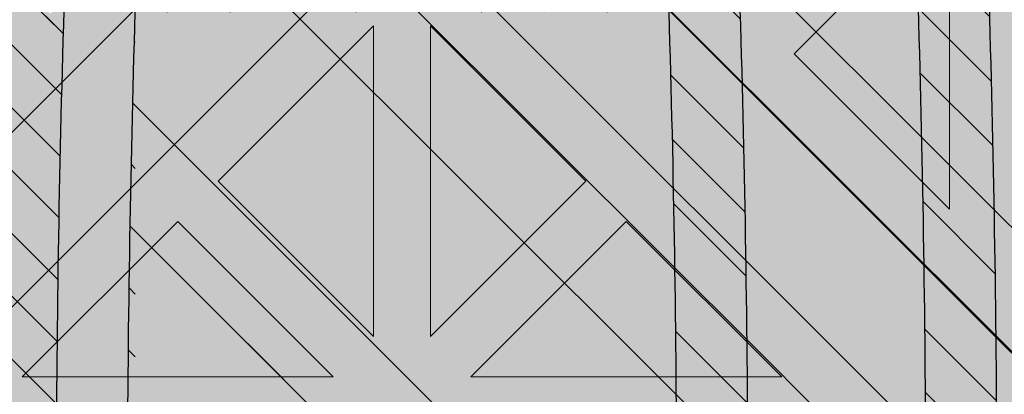
# Model space of a CAD drawing. Units: inches. Extents: x 844 to 2234, y 346 to 1084.
# Tile 32 of 93: x 1255.662 to 1260.074, y 698.789 to 700.469. Entities that reach past the tile are written whole.
import ezdxf

# ---------------------------------------------------------------- set-up
doc = ezdxf.new("R2010")
doc.units = ezdxf.units.IN
doc.header["$MEASUREMENT"] = 0
doc.layers.add('furniture', color=8, linetype='Continuous', lineweight=18)
doc.layers.add('RA-AP-01$0$INT', color=35, linetype='Continuous', lineweight=5)
doc.layers.add('RA-AP-01$0$FURN', color=3, linetype='Continuous')
doc.layers.add('RA-AP-01$0$WOOD', color=64, linetype='Continuous')

# ---------------------------------------------------------------- blocks, each defined once
blk = doc.blocks.new('A$C18D01794')
at = {"layer": 'RA-AP-01$0$INT'}
h = blk.add_hatch(color=256, dxfattribs=at)
h.paths.add_polyline_path([(4.585917135068448, -7.856712009587804), (4.614201406330596, -7.856712009587056), (4.668846067270487, -7.802067348644738), (4.723490728212344, -7.856712009584164), (4.771774999457151, -7.856712009582887), (4.826419660396886, -7.80206734864072), (4.862780050090322, -7.838427738332541), (4.844495778842715, -7.856712009580965), (4.862780050090411, -7.856712009580482), (4.905206456960182, -7.814285602707865), (4.947632863832445, -7.856712009578238), (4.965917135079675, -7.856712009577755), (4.947632863831759, -7.838427738330656), (4.983993253523576, -7.802067348637219), (5.038637914464627, -7.856712009575829), (5.08692218571208, -7.856712009574554), (5.141566846649976, -7.802067348634224), (5.196211507589851, -7.856712009571666), (5.224495778822615, -7.856712009570916), (4.905206456953975, -7.537422687702283)])
h.paths.add_polyline_path([(4.895206456956031, -7.575706958950402), (4.895206456958921, -7.684996280828174), (4.840561796018589, -7.630351619890275)], flags=16)
h.paths.add_polyline_path([(4.915206456955638, -7.575706958949956), (4.969851117895509, -7.630351619887399), (4.915206456957609, -7.684996280827732)], flags=16)
h.paths.add_polyline_path([(4.826419660395175, -7.644493755514321), (4.881064321335613, -7.699138416452331), (4.771774999456703, -7.69913841645522)], flags=16)
h.paths.add_polyline_path([(4.983993253519558, -7.644493755510815), (5.038637914460456, -7.699138416449285), (4.929348592581548, -7.69913841645126)], flags=16)
h.paths.add_polyline_path([(4.881064321336025, -7.719138416452334), (4.826419660397532, -7.773783077393256), (4.771774999457062, -7.719138416455217)], flags=16)
h.paths.add_polyline_path([(4.929348592582019, -7.71913841645126), (5.038637914460982, -7.719138416449284), (4.983993253522945, -7.773783077389749)], flags=16)
h.paths.add_polyline_path([(4.895206456960191, -7.733280552075633), (4.895206456962115, -7.806001331460164), (4.876922185715016, -7.824285602708492), (4.840561796021581, -7.787925213016675)], flags=16)
h.paths.add_polyline_path([(4.915206456958487, -7.733280552075187), (4.969851117899527, -7.787925213013798), (4.933490728206909, -7.824285602708034), (4.9152064569598, -7.806001331461736)], flags=16)
h.paths.add_polyline_path([(4.757632863832376, -7.733280552079264), (4.812277524772842, -7.787925213017304), (4.757632863834348, -7.842569873958233)], flags=16)
h.paths.add_polyline_path([(4.737632863832376, -7.73328055207979), (4.737632863834348, -7.842569873958701), (4.682988202893906, -7.787925213020692)], flags=16)
h.paths.add_polyline_path([(5.05278005008503, -7.733280552072701), (5.052780050087917, -7.842569873951664), (4.998135389146995, -7.787925213013169)], flags=16)
h.paths.add_polyline_path([(5.072780050085024, -7.733280552072333), (5.127424711025931, -7.787925213010806), (5.072780050087916, -7.842569873951244)], flags=16)
h.paths.add_polyline_path([(4.935917135072783, -7.506712009583784), (5.255206456948811, -7.826001331459767), (5.255206456948932, -7.797717060211899), (5.200561796010279, -7.743072399273238), (5.255206456949403, -7.688427738334128), (5.25520645694961, -7.640143467086677), (5.200561796009787, -7.585498806146837), (5.236922185702417, -7.549138416454212), (5.255206456949919, -7.56742268770172), (5.255206456949998, -7.549138416454178), (5.212780050078687, -7.506712009583814), (5.25520645695036, -7.464285602712145), (5.255206456950438, -7.446001331464763), (5.236922185702424, -7.464285602712779), (5.200561796009796, -7.427925213020149), (5.255206456950753, -7.373280552079203), (5.25520645695096, -7.324996280834394), (5.200561796010322, -7.270351619893748), (5.255206456951428, -7.215706958952649), (5.255206456951547, -7.187422687705071)])
h.paths.add_polyline_path([(5.042988202883395, -7.42792521302065), (5.097632863823085, -7.373280552080975), (5.097632863822622, -7.482569873959883)], flags=16)
h.paths.add_polyline_path([(5.028846067259663, -7.442067348644384), (5.083490728198774, -7.496712009583504), (4.974201406321001, -7.496712009583035)], flags=16)
h.paths.add_polyline_path([(5.117632863823087, -7.37328055208089), (5.172277524762331, -7.42792521302015), (5.11763286382262, -7.482569873959851)], flags=16)
h.paths.add_polyline_path([(5.08349072819877, -7.516712009582191), (5.028846067259652, -7.571356670521302), (4.974201406320998, -7.516712009582638)], flags=16)
h.paths.add_polyline_path([(5.131774999446817, -7.35913841645716), (5.186419660386065, -7.413783077396415), (5.241064321325782, -7.359138416456712)], flags=17)
h.paths.add_polyline_path([(5.131774999446228, -7.496712009583703), (5.186419660386065, -7.442067348643883), (5.222780050079488, -7.478427738337313), (5.204495778832781, -7.496712009584014)], flags=16)
h.paths.add_polyline_path([(5.097632863822613, -7.530854145205813), (5.097632863823061, -7.640143467084723), (5.042988202883383, -7.585498806145032)], flags=16)
h.paths.add_polyline_path([(5.131774999446899, -7.339138416457162), (5.241064321325809, -7.339138416456712), (5.186419660386591, -7.284493755517479)], flags=17)
h.paths.add_polyline_path([(5.131774999446226, -7.516712009581999), (5.204495778830767, -7.516712009581702), (5.22278005007868, -7.534996280829206), (5.186419660386049, -7.571356670521828)], flags=16)
h.paths.add_polyline_path([(5.11763286382262, -7.530854145205852), (5.17227752476232, -7.585498806145562), (5.117632863823064, -7.64014346708481)], flags=16)
h.paths.add_polyline_path([(5.186419660386069, -7.599640941770585), (5.241064321325754, -7.654285602710281), (5.131774999446791, -7.654285602709814)], flags=16)
h.paths.add_polyline_path([(5.131774999446872, -7.674285602709813), (5.24106432132578, -7.674285602710282), (5.186419660386554, -7.728930263649504)], flags=16)
h.paths.add_polyline_path([(5.255206456951811, -7.126001331467467), (5.255206456951895, -7.106712009588038), (4.555206456956052, -7.106712009588038), (4.555206456956136, -7.12600133146746), (4.905206456953973, -7.476001331465289)])
h.paths.add_polyline_path([(4.983993253513404, -7.368930263651977), (4.92934859257295, -7.314285602713969), (5.03863791445186, -7.314285602711063)], flags=16)
h.paths.add_polyline_path([(4.969851117889988, -7.383072399276016), (4.915206456952556, -7.437717060215906), (4.915206456949648, -7.328427738338133)], flags=16)
h.paths.add_polyline_path([(4.929348592572535, -7.294285602713971), (4.983993253511019, -7.239640941773039), (5.038637914451496, -7.294285602711065)], flags=16)
h.paths.add_polyline_path([(5.052780050074912, -7.280143467087016), (4.998135389134438, -7.225498806148989), (5.052780050072919, -7.170854145208052)], flags=16)
h.paths.add_polyline_path([(5.07278005007491, -7.280143467086489), (5.072780050072918, -7.170854145207579), (5.127424711013374, -7.225498806145578)], flags=16)
h.paths.add_polyline_path([(4.89520645695295, -7.437717060216355), (4.840561796013067, -7.383072399278919), (4.895206456950961, -7.328427738338582)], flags=16)
h.paths.add_polyline_path([(4.915206456948365, -7.280143467090674), (4.915206456946434, -7.207422687704125), (4.933490728192729, -7.18913841645701), (4.969851117886972, -7.225498806149623)], flags=16)
h.paths.add_polyline_path([(4.881064321327021, -7.314285602715054), (4.82641966038902, -7.368930263655506), (4.771774999448108, -7.314285602717047)], flags=16)
h.paths.add_polyline_path([(4.895206456950073, -7.280143467091125), (4.840561796009022, -7.225498806152518), (4.876922185700835, -7.18913841645908), (4.895206456948749, -7.207422687706589)], flags=16)
h.paths.add_polyline_path([(4.983993253510392, -7.211356670525576), (4.947632863816944, -7.174996280833758), (4.965917135064043, -7.156712009585847), (5.038637914448995, -7.156712009584522)], flags=16)
h.paths.add_polyline_path([(4.881064321326543, -7.294285602715056), (4.771774999447578, -7.294285602717046), (4.826419660385607, -7.239640941776569)], flags=16)
h.paths.add_polyline_path([(4.905206456946447, -7.19913841645844), (4.862780050074785, -7.156712009587725), (4.947632863816685, -7.156712009586302)], flags=16)
h.paths.add_polyline_path([(5.14156684663679, -7.211356670521528), (5.086922185696452, -7.156712009583639), (5.196211507574223, -7.156712009581651)], flags=16)
h.paths.add_polyline_path([(4.8264196603837, -7.211356670529104), (4.771774999442643, -7.156712009590501), (4.8444957788276, -7.156712009588568), (4.862780050075511, -7.17499628083566)], flags=16)
h.paths.add_polyline_path([(4.812277524760289, -7.225498806153156), (4.757632863822258, -7.28014346709363), (4.757632863819352, -7.170854145214669)], flags=16)
h.paths.add_polyline_path([(4.73763286382226, -7.280143467093997), (4.682988202881349, -7.22549880615554), (4.737632863819352, -7.170854145215086)], flags=16)
h.paths.add_polyline_path([(4.723490728195188, -7.156712009591787), (4.668846067257299, -7.211356670532127), (4.614201406317417, -7.156712009594693)], flags=16)
h.paths.add_polyline_path([(4.597632863829262, -7.506712009583814), (4.555206456957951, -7.54913841645418), (4.555206456958029, -7.56742268770172), (4.573490728205535, -7.549138416454212), (4.609851117898167, -7.585498806146839), (4.555206456958338, -7.640143467086675), (4.555206456958546, -7.688427738334125), (4.60985111789767, -7.743072399273238), (4.555206456959015, -7.797717060211899), (4.555206456959138, -7.826001331459767), (4.874495778835167, -7.506712009583786), (4.5552064569564, -7.187422687705062), (4.555206456956523, -7.215706958952644), (4.609851117897629, -7.270351619893746), (4.555206456956988, -7.324996280834396), (4.555206456957198, -7.373280552079195), (4.609851117898153, -7.427925213020147), (4.573490728205528, -7.464285602712779), (4.555206456957507, -7.446001331464756), (4.555206456957585, -7.464285602712143)])
h.paths.add_polyline_path([(4.712780050085332, -7.482569873959882), (4.712780050084863, -7.373280552080972), (4.767424711024555, -7.42792521302065)], flags=16)
h.paths.add_polyline_path([(4.726922185709173, -7.496712009583504), (4.781566846648288, -7.442067348644384), (4.836211507586949, -7.496712009583033)], flags=16)
h.paths.add_polyline_path([(4.692780050085327, -7.482569873959851), (4.638135389145619, -7.427925213020149), (4.692780050084865, -7.373280552080892)], flags=16)
h.paths.add_polyline_path([(4.726922185709182, -7.516712009582191), (4.836211507586949, -7.51671200958264), (4.7815668466483, -7.571356670521304)], flags=16)
h.paths.add_polyline_path([(4.678637914461726, -7.496712009583706), (4.605917135075169, -7.496712009584014), (4.587632863828464, -7.478427738337311), (4.623993253521887, -7.442067348643881)], flags=16)
h.paths.add_polyline_path([(4.712780050085336, -7.530854145205816), (4.767424711024568, -7.585498806145034), (4.71278005008489, -7.640143467084724)], flags=16)
h.paths.add_polyline_path([(4.678637914461726, -7.516712009582001), (4.623993253521899, -7.571356670521829), (4.587632863829271, -7.534996280829206), (4.605917135077185, -7.5167120095817)], flags=16)
h.paths.add_polyline_path([(4.692780050085336, -7.530854145205848), (4.692780050084889, -7.64014346708481), (4.638135389145632, -7.585498806145562)], flags=16)
h.paths.add_polyline_path([(4.623993253521885, -7.413783077396415), (4.678637914461131, -7.359138416457161), (4.56934859258217, -7.359138416456712)], flags=17)
h.paths.add_polyline_path([(4.623993253521901, -7.599640941770568), (4.678637914461158, -7.654285602709814), (4.569348592582195, -7.654285602710281)], flags=16)
h.paths.add_polyline_path([(4.678637914461051, -7.339138416457162), (4.623993253521361, -7.284493755517479), (4.569348592582143, -7.339138416456712)], flags=17)
h.paths.add_polyline_path([(4.678637914461076, -7.674285602709813), (4.623993253521399, -7.728930263649504), (4.569348592582167, -7.674285602710281)], flags=16)
h = blk.add_hatch(color=256, dxfattribs=at)
h.paths.add_polyline_path([(4.905206456954232, -7.537422687702028), (4.874495778835232, -7.506712009583718), (4.555206456959138, -7.826001331459766), (4.555206456959269, -7.856712009588616), (4.585917135068449, -7.856712009587804)])
h.paths.add_polyline_path([(4.935917135072152, -7.506712009583152), (4.905206456953497, -7.537422687701806), (5.224495778822614, -7.856712009570917), (5.255206456948681, -7.856712009570104), (5.255206456948813, -7.826001331459768)])
h.paths.add_polyline_path([(5.255206456951549, -7.18742268770507), (5.255206456951813, -7.126001331467461), (4.905206456953563, -7.476001331465701), (4.935917135072559, -7.506712009584006)])
h.paths.add_polyline_path([(4.874495778835167, -7.506712009583785), (4.905206456953818, -7.476001331465132), (4.555206456956135, -7.126001331467458), (4.555206456956399, -7.187422687705064)])
h = blk.add_hatch(color=256, dxfattribs=at)
h.paths.add_polyline_path([(4.89520645695096, -7.328427738338579), (4.840561796013068, -7.383072399278921), (4.89520645695295, -7.437717060216353)])
h.paths.add_polyline_path([(4.915206456952557, -7.437717060215907), (4.969851117889986, -7.383072399276024), (4.915206456949648, -7.328427738338133)])
h.paths.add_polyline_path([(4.929348592572952, -7.31428560271397), (4.983993253513403, -7.368930263651974), (5.038637914451863, -7.314285602711064)])
h.paths.add_polyline_path([(5.038637914451498, -7.294285602711065), (4.983993253511018, -7.239640941773039), (4.929348592572535, -7.294285602713969)])
h.paths.add_polyline_path([(4.969851117886971, -7.225498806149624), (4.93349072819273, -7.189138416457011), (4.915206456946433, -7.207422687704124), (4.915206456948367, -7.280143467090678)])
h.paths.add_polyline_path([(4.965917135064045, -7.156712009585847), (4.947632863816945, -7.17499628083376), (4.983993253510389, -7.211356670525573), (5.038637914448995, -7.156712009584522)])
h.paths.add_polyline_path([(4.998135389134439, -7.22549880614899), (5.05278005007491, -7.280143467087016), (5.052780050072921, -7.170854145208054)])
h.paths.add_polyline_path([(5.072780050074911, -7.28014346708649), (5.127424711013374, -7.225498806145579), (5.072780050072921, -7.170854145207581)])
h.paths.add_polyline_path([(5.196211507574225, -7.156712009581651), (5.08692218569645, -7.156712009583639), (5.141566846636789, -7.211356670521529)])
h.paths.add_polyline_path([(4.862780050074782, -7.156712009587723), (4.90520645694645, -7.199138416458444), (4.94763286381669, -7.156712009586302)])
h.paths.add_polyline_path([(4.895206456950073, -7.280143467091126), (4.895206456948746, -7.207422687706587), (4.876922185700836, -7.189138416459078), (4.840561796009025, -7.225498806152521)])
h.paths.add_polyline_path([(4.826419660385605, -7.239640941776569), (4.771774999447577, -7.294285602717049), (4.881064321326541, -7.294285602715055)])
h.paths.add_polyline_path([(4.771774999448108, -7.314285602717046), (4.82641966038902, -7.368930263655505), (4.88106432132702, -7.314285602715054)])
h.paths.add_polyline_path([(4.757632863822258, -7.280143467093631), (4.812277524760285, -7.225498806153153), (4.757632863819352, -7.170854145214668)])
h.paths.add_polyline_path([(4.862780050075512, -7.17499628083566), (4.844495778827599, -7.156712009588567), (4.771774999442647, -7.156712009590504), (4.8264196603837, -7.211356670529104)])
h.paths.add_polyline_path([(4.682988202881349, -7.225498806155537), (4.737632863822258, -7.280143467093997), (4.737632863819352, -7.170854145215087)])
h.paths.add_polyline_path([(4.723490728195189, -7.156712009591783), (4.614201406317418, -7.156712009594692), (4.668846067257298, -7.211356670532127)])
h = blk.add_hatch(color=256, dxfattribs=at)
h.paths.add_polyline_path([(4.781566846647504, -7.442067348645805), (4.836211507586161, -7.496712009584463), (4.726922185708388, -7.496712009584918)])
h.paths.add_polyline_path([(4.836211507586161, -7.516712009584068), (4.781566846647504, -7.571356670522723), (4.726922185708388, -7.516712009583606)])
h.paths.add_polyline_path([(4.76742471102377, -7.585498806146453), (4.712780050084083, -7.640143467086137), (4.712780050084542, -7.530854145207227)])
h.paths.add_polyline_path([(4.692780050084544, -7.530854145207257), (4.692780050084084, -7.64014346708622), (4.638135389144834, -7.585498806146965)])
h.paths.add_polyline_path([(4.678637914460932, -7.516712009583407), (4.623993253521102, -7.571356670523233), (4.587632863827676, -7.53499628082981), (4.605917135074382, -7.516712009583104)])
h.paths.add_polyline_path([(4.573490728204743, -7.54913841645434), (4.60985111789737, -7.585498806146969), (4.555206456957541, -7.640143467086797), (4.555206456957237, -7.567422687701846)])
h.paths.add_polyline_path([(4.623993253521098, -7.599640941770699), (4.67863791446035, -7.654285602709951), (4.56934859258139, -7.654285602710407)])
h.paths.add_polyline_path([(4.678637914460275, -7.67428560270995), (4.623993253520583, -7.728930263649637), (4.56934859258136, -7.674285602710405)])
h.paths.add_polyline_path([(4.609851117896854, -7.743072399273369), (4.555206456958196, -7.797717060212026), (4.555206456957738, -7.688427738334254)])
h.paths.add_polyline_path([(4.597632863828475, -7.506712009583301), (4.555206456957283, -7.549138416454495), (4.555206456956805, -7.464285602712587)])
h.paths.add_polyline_path([(4.678637914460932, -7.496712009585113), (4.605917135076396, -7.496712009585417), (4.587632863828479, -7.478427738337913), (4.623993253521104, -7.442067348645284)])
h.paths.add_polyline_path([(4.692780050084091, -7.373280552082301), (4.692780050084548, -7.482569873961267), (4.638135389144834, -7.427925213021552)])
h.paths.add_polyline_path([(4.767424711023772, -7.427925213022072), (4.712780050084545, -7.48256987396129), (4.712780050084089, -7.373280552082384)])
h.paths.add_polyline_path([(4.67863791446036, -7.359138416457298), (4.623993253521105, -7.41378307739655), (4.569348592581399, -7.35913841645684)])
h.paths.add_polyline_path([(4.609851117897371, -7.427925213020278), (4.573490728204743, -7.464285602712907), (4.555206456957237, -7.446001331465401), (4.555206456957548, -7.373280552080448)])
h.paths.add_polyline_path([(4.623993253520596, -7.284493755517612), (4.67863791446028, -7.339138416457299), (4.569348592581367, -7.339138416456838)])
h.paths.add_polyline_path([(4.609851117896867, -7.270351619893878), (4.555206456957749, -7.324996280832994), (4.55520645695821, -7.21570695895522)])
for p, q in [((4.905206456953975, -7.476001331465289), (4.555206456956136, -7.12600133146746)), ((4.905206456953975, -7.476001331465289), (5.255206456951811, -7.126001331467465)), ((4.874495778835167, -7.506712009583786), (4.555206456956399, -7.187422687705064)), ((4.935917135072783, -7.506712009583784), (5.255206456951548, -7.187422687705069)), ((4.771774999448109, -7.314285602717045), (4.881064321327019, -7.314285602715054)), ((4.826419660389018, -7.368930263655503), (4.771774999448109, -7.314285602717045)), ((4.881064321327019, -7.314285602715054), (4.82641966038902, -7.368930263655505)), ((4.929348592572952, -7.314285602713971), (4.983993253513403, -7.368930263651975)), ((5.038637914451862, -7.314285602711064), (4.929348592572952, -7.314285602713971)), ((4.983993253513404, -7.368930263651973), (5.038637914451862, -7.314285602711064)), ((4.895206456950956, -7.328427738338584), (4.840561796013068, -7.383072399278921)), ((4.895206456950959, -7.328427738338582), (4.89520645695295, -7.437717060216353)), ((4.915206456949651, -7.328427738338136), (4.969851117889986, -7.383072399276024)), ((4.915206456949648, -7.328427738338135), (4.915206456952556, -7.437717060215906)), ((4.767424711024554, -7.42792521302065), (4.712780050084865, -7.373280552080972)), ((4.712780050084865, -7.373280552080972), (4.71278005008533, -7.482569873959882)), ((4.89520645695295, -7.437717060216353), (4.840561796013068, -7.383072399278921)), ((4.915206456952556, -7.437717060215906), (4.969851117889986, -7.383072399276024)), ((4.71278005008533, -7.482569873959882), (4.767424711024555, -7.427925213020651))]:
    blk.add_line(p, q, dxfattribs=at)
blk = doc.blocks.new('A$C32926AE1')
at = {"layer": 'RA-AP-01$0$FURN'}
h = blk.add_hatch(dxfattribs=at)
h.set_pattern_fill('ANSI31', color=256, scale=0.1, style=0)
h.set_pattern_definition([(45, (0, 0), (-0.0088388347648318, 0.0088388347648318), [])])
edge = h.paths.add_edge_path(flags=16)
edge.add_arc((4.904771284329206, 4.246793130718756), 0.2603971832811541, 75.22398030683196, 104.7760196931204)
edge.add_arc((4.904771284329206, 4.246793130718756), 0.2603971832811541, 75.223980306832, 104.77601969312039, ccw=False)
edge = h.paths.add_edge_path(flags=16)
edge.add_arc((4.904771284329206, 4.067062675376612), 0.2603971832811541, 255.2239803068796, 284.776019693168)
edge.add_arc((4.904771284329206, 4.067062675376612), 0.2603971832811541, 255.22398030687958, 284.77601969316805, ccw=False)
edge = h.paths.add_edge_path(flags=0)
edge.add_arc((4.904771284329206, 4.067062675376612), 0.2603971832811541, 255.2239803068796, 284.776019693168)
edge.add_arc((4.904771284329206, 4.067062675376612), 0.2603971832811541, 255.22398030687958, 284.77601969316805, ccw=False)
edge = h.paths.add_edge_path(flags=0)
edge.add_arc((4.904771284329206, 4.067062675376612), 0.2603971832811541, 255.2239803068796, 284.776019693168)
edge.add_arc((4.904771284329206, 4.067062675376612), 0.2603971832811541, 255.22398030687958, 284.77601969316805, ccw=False)
edge = h.paths.add_edge_path()
edge.add_arc((4.604388392048174, 4.588829985554312), 0.1599999999999918, 342.3781640246255, 354.4317409793762)
edge.add_arc((5.090145208887507, 4.43216705527679), 0.3503971832811637, 162.0091218307731, 180.3186872093483)
edge.add_arc((5.205154176610243, 4.588829985554953), 0.1599999999999917, 185.5682590208461, 197.6218359767349)
edge.add_arc((4.904771284329229, 4.246793130718735), 0.3503971832811761, 72.00912183053516, 107.9908781690354)
edge.add_arc((9.535952835716557, 4.28682295566602), 4.798342501046485, 178.2875002453811, 181.5576802719453)
edge.add_arc((4.719397359771122, 4.43216705527679), 0.3503971832811637, 359.6813127906516, 377.9908781692269)
edge.add_arc((9.535967292294904, 4.286822350292874), 4.778371420254705, 178.2965938931842, 181.5667745797229)
edge.add_arc((4.719397359771122, 4.43216705527679), 0.3303971832811637, 359.6813127906516, 377.9908781692269)
edge.add_arc((0.2735752763637294, 4.286822350292874), 4.7783714202547, 358.4332254202771, 361.7034061068158)
edge.add_arc((5.061434214606998, 4.732549947558029), 0.1600000000000254, 252.3781640250584, 264.4317409792362)
edge.add_arc((4.748108354051257, 4.732549947558012), 0.1600000000000541, 275.5682590208426, 287.6218359759532)
edge.add_arc((4.604388392048115, 4.588829985554317), 0.1800000000000505, 342.3567572500182, 349.3735009646207)
edge.add_arc((5.205154176610254, 4.588829985554976), 0.1800000000000069, 190.6264990356027, 197.6432427513933)
edge.add_arc((5.061434214607106, 4.732549947558013), 0.1800000000000424, 252.3567572496606, 259.3735009644582)
edge.add_arc((4.904771284329208, 4.246793130718737), 0.3303971832811676, 71.99844483668534, 108.0015551637021)
edge.add_arc((4.748108354051414, 4.732549947558045), 0.1800000000000547, 280.6264990355479, 287.6432427495938)
edge.add_arc((5.090145208887514, 4.432167055276789), 0.2803971832811691, 162.8706300666893, 180.816523289902)
edge.add_arc((4.719397359771136, 4.432167055276689), 0.2803971832811534, 359.183476710103, 377.1293699333214)
edge.add_arc((4.904771284329222, 4.246793130718737), 0.2803971832811769, 72.87063006672916, 107.1293699332334)
edge.add_arc((5.090145208887522, 4.432167055276788), 0.2603971832811776, 165.2239803068007, 180.9953123810312)
edge.add_arc((4.719397359771141, 4.432167055276699), 0.2603971832811458, 359.0046876189768, 374.7760196932087)
edge.add_arc((5.090145208887507, 4.43216705527679), 0.3303971832811637, 162.0091218307731, 180.3186872093483)
edge.add_arc((9.53595427642584, 4.285015535491528), 4.728345371032053, 178.265043920078, 181.5679956281801)
edge.add_arc((0.2735882922327999, 4.285015535491582), 4.728345371032045, 358.4320043718193, 361.7349560799204)
edge.add_arc((9.535953591267507, 4.284458026472751), 4.708343996644348, 178.2573054306777, 181.5704995759608)
edge.add_arc((0.273588977391114, 4.284458026472785), 4.708343996644358, 358.4295004240388, 361.7426945693213)
edge.add_arc((0.2735889773911131, 4.029397779622582), 4.708343996644359, 358.2573054306787, 361.5704995759613)
edge.add_arc((9.535953591267518, 4.029397779622618), 4.708343996644359, 178.4295004240391, 181.7426945693223)
edge.add_arc((0.2735882922327901, 4.028840270603786), 4.728345371032054, 358.2650439200796, 361.5679956281808)
edge.add_arc((9.53595427642584, 4.028840270603841), 4.728345371032054, 178.4320043718199, 181.7349560799219)
edge.add_arc((0.2735752763637302, 4.027033455802493), 4.778371420254699, 358.2965938931842, 361.5667745797229)
edge.add_arc((4.719397359771122, 3.881688750818578), 0.3303971832811637, 342.0091218307731, 360.3186872093484)
edge.add_arc((5.090145208887507, 3.881688750818578), 0.3303971832811637, 179.6813127906516, 197.9908781692269)
edge.add_arc((9.535967292294904, 4.027033455802493), 4.778371420254705, 178.433225420277, 181.7034061068158)
edge.add_arc((4.719397359771122, 3.881688750818578), 0.3503971832811637, 342.0091218307731, 360.3186872093484)
edge.add_arc((9.53595283571655, 4.027032850429349), 4.79834250104648, 178.4423197280546, 181.7124997546188)
edge.add_arc((4.719397359771141, 3.881688750818669), 0.2603971832811458, 345.2239803067913, 360.9953123810232)
edge.add_arc((5.090145208887522, 3.88168875081858), 0.2603971832811776, 179.0046876189687, 194.7760196931993)
edge.add_arc((4.904771284329222, 4.067062675376631), 0.2803971832811769, 252.8706300667665, 287.1293699332708)
edge.add_arc((4.719397359771136, 3.881688750818678), 0.2803971832811534, 342.8706300666787, 360.8165232898969)
edge.add_arc((5.090145208887514, 3.881688750818579), 0.2803971832811691, 179.183476710098, 197.1293699333106)
edge.add_arc((4.748108354051414, 3.581305858537323), 0.1800000000000547, 72.3567572504062, 79.37350096445199)
edge.add_arc((4.904771284329208, 4.067062675376631), 0.3303971832811676, 251.9984448362979, 288.0015551633146)
edge.add_arc((5.061434214607106, 3.581305858537355), 0.1800000000000424, 100.6264990355418, 107.6432427503394)
edge.add_arc((5.205154176610254, 3.725025820540392), 0.1800000000000069, 162.3567572486066, 169.3735009643972)
edge.add_arc((4.604388392048115, 3.725025820541051), 0.1800000000000505, 10.62649903537925, 17.64324274998182)
edge.add_arc((4.748108354051257, 3.581305858537356), 0.1600000000000541, 72.37816402404681, 84.43174097915735)
edge.add_arc((4.904771284329229, 4.067062675376632), 0.3503971832811761, 252.0091218309645, 287.9908781694648)
edge.add_arc((5.061434214606998, 3.581305858537339), 0.1600000000000254, 95.56825902076373, 107.6218359749416)
edge.add_arc((5.205154176610243, 3.725025820540414), 0.1599999999999917, 162.3781640232651, 174.4317409791539)
edge.add_arc((5.090145208887507, 3.881688750818578), 0.3503971832811637, 179.6813127906516, 197.9908781692269)
edge.add_arc((4.604388392048174, 3.725025820541056), 0.1599999999999918, 5.568259020623824, 17.62183597537444)
edge.add_arc((0.2735897329420762, 4.28682295566602), 4.798342501046482, 358.4423197280547, 361.7124997546188)
edge.add_arc((0.2735897329420691, 4.027032850429348), 4.798342501046489, 358.2875002453812, 361.5576802719453)
at = {"layer": 'RA-AP-01$0$WOOD'}
h = blk.add_hatch(color=256, dxfattribs=at)
h.dxf.hatch_style = 1
h.paths.add_polyline_path([(5.157430609644524, 4.573483066760929, -0.1009492694046607), (5.155401577623758, 4.593365984175333, -0.1842662638101597), (5.172249623284174, 4.638795604568598, 0.2056608120311276), (5.179560981299304, 4.661316324430096, 0.3614336704623542), (5.134352340494423, 4.706524965234944, 0.2056608120311297), (5.111831620632933, 4.699213607219793, -0.1842662638101113), (5.066402000239693, 4.682365561559342, -0.1055311479399994), (5.045656153913092, 4.68467289944697, 0.1567636581983829), (4.763886414745334, 4.684672899446966, -0.1055311479399895), (4.743140568418733, 4.68236556155934, -0.1842662638100833), (4.6977109480255, 4.69921360721979, 0.2056608120302612), (4.675190228164109, 4.706524965234949, 0.3614336704708441), (4.629981587358889, 4.66131632442871, 0.2056608120245944), (4.637292945374126, 4.638795604567974, -0.1842662638101024), (4.654140991034615, 4.59336598417475, -0.1009492694055169), (4.652111959013835, 4.573483066760181, 0.021410119221476), (4.629748025606143, 4.156712009541676, 0.0214101192214795), (4.652111959013809, 3.739940952323101, -0.1009492694059586), (4.654140991034615, 3.720058034908448, -0.1842662638100975), (4.637292945374126, 3.674628414515226, 0.2056608120245705), (4.629981587358889, 3.652107694654492, 0.3614336704708879), (4.675190228164113, 3.606899053848249, 0.2056608120302384), (4.697710948025501, 3.614210411863408, -0.1842662638100995), (4.743140568418738, 3.63105845752386, -0.1055311479402541), (4.763886414745388, 3.628751119636215, 0.1567636581983776), (5.045656153913137, 3.628751119636244, -0.1055311479397538), (5.066402000239692, 3.631058457523857, -0.1842662638101067), (5.111831620632931, 3.614210411863407, 0.2056608120310924), (5.134352340494417, 3.606899053848256, 0.3614336704624001), (5.179560981299307, 3.652107694653103, 0.2056608120311314), (5.172249623284175, 3.6746284145146, -0.1842662638101402), (5.155401577623758, 3.72005803490786, -0.1009492694051366), (5.15743060964455, 3.739940952322354, 0.0214101192215073), (5.179794543052287, 4.156712009541468, 0.0214101192215252)])
h.paths.add_polyline_path([(4.639748609479751, 4.156712009541513, 0.0213537860821624), (4.661970494867118, 3.741887061152232, -0.094075836301374), (4.664143710413708, 3.7196126951003, -0.1824818158568985), (4.644813765429836, 3.668037719127816, 0.2056608120245319), (4.639939526753007, 3.653023905887301, 0.3614336704710246), (4.676106439397173, 3.616856993242342, 0.2056608120302234), (4.691120252638095, 3.621731231919122, -0.1824818158602558), (4.742695228611606, 3.641061176902986, -0.1029891339458722), (4.766991894714349, 3.638256818950944, 0.156709409989566), (5.042550673941472, 3.638256818950105, -0.102989133958497), (5.066847340047078, 3.641061176902949, -0.1824818158594995), (5.118422316020358, 3.621731231919103, 0.2056608120311416), (5.133436129261316, 3.616856993242346, 0.3614336704621468), (5.169603041905217, 3.653023905886178, 0.2056608120310986), (5.164728803228477, 3.668037719127177, -0.1824818158565612), (5.145398858244737, 3.719612695099578, -0.0940758363009313), (5.147572073791232, 3.741887061151398, 0.0213537860822023), (5.169793959178681, 4.156712009541451, 0.0213537860822226), (5.147572073791203, 4.571536957931898, -0.0940758363005034), (5.145398858244737, 4.59381132398362, -0.1824818158565587), (5.164728803228476, 4.645386299956021, 0.2056608120311045), (5.169603041905216, 4.66040011319702, 0.3614336704621845), (5.133436129261313, 4.696567025840856, 0.2056608120310773), (5.118422316020359, 4.691692787164098, -0.182481815859508), (5.066847340047078, 4.67236284218025, -0.1029891339584606), (5.04255067394148, 4.675167200133092, 0.156709409989566), (4.766991894714357, 4.675167200132257, -0.1029891339458842), (4.742695228611611, 4.672362842180213, -0.1824818158602725), (4.691120252638095, 4.691692787164077, 0.2056608120302152), (4.676106439397174, 4.696567025840858, 0.3614336704710363), (4.639939526753005, 4.660400113195899, 0.2056608120245495), (4.644813765429837, 4.645386299955384, -0.1824818158568934), (4.664143710413708, 4.593811323982902, -0.0940758363009187), (4.661970494867149, 4.571536957931074, 0.021353786082177)], flags=16)
h.paths.add_polyline_path([(5.129794543052235, 4.432167055276933, -0.0141661062790638), (5.130152669293814, 4.156927903047693, -0.0141661062790647), (5.129794543052234, 3.881688750818433, -0.0785247771143638), (5.10979738006795, 3.755143611847103, 0.0945969212073497), (5.105408519571111, 3.717898134952927, 0.1043170707844957), (5.116074640131521, 3.670385395016088, 0.1043170707864965), (5.068561900193738, 3.681051515576561, 0.09459692119553), (5.031316423304057, 3.676662655080835, -0.1580239521427272), (4.778226145355827, 3.676662655080367, 0.0945969211986668), (4.740980668464973, 3.681051515576592, 0.1043170707882822), (4.693467928526415, 3.670385395015844, 0.1043170707867916), (4.704134049087309, 3.717898134953662, 0.0945969211972894), (4.69974518859162, 3.755143611844042, -0.0785247771163196), (4.679748025606343, 3.881688750818406, -0.0141661062790663), (4.679389899364763, 4.156927903047693, -0.0141661062790672), (4.679748025606343, 4.432167055276998, -0.0785247771163064), (4.699745188591625, 4.55871219425134, 0.094596921197333), (4.704134049087308, 4.595957671141738, 0.1043170707867205), (4.693467928526416, 4.643470411079523, 0.1043170707882628), (4.740980668464965, 4.632804290518776, 0.0945969211988114), (4.778226145355874, 4.637193151015016, -0.158023952142669), (5.031316423304015, 4.637193151014546, 0.0945969211956361), (5.068561900193736, 4.632804290518806, 0.1043170707864979), (5.11607464013152, 4.643470411079278, 0.1043170707844617), (5.105408519571112, 4.595957671142455, 0.0945969212074597), (5.109797380067959, 4.558712194248236, -0.0785247771143467)], flags=0)
h.paths.add_polyline_path([(5.119794532311105, 4.432259799204851, -0.0142000800617244), (5.120156169157484, 4.156927903047701, -0.0142000800617277), (5.119794532311105, 3.881596006890482, -0.0784894509520253), (5.100273383573699, 3.758192358677797, 0.0940138827242913), (5.095413455884425, 3.717477693979438, 0.0606271852308753), (5.099615656341024, 3.686844378806616, 0.0606271852322524), (5.068982341167493, 3.691046579263239, 0.0940138827010453), (5.028267676478798, 3.686186651576848, -0.1580706864508061), (4.781274892180912, 3.686186651576435, 0.0940138827026903), (4.740560227491556, 3.691046579263279, 0.0606271852339895), (4.709926912317155, 3.686844378806508, 0.0606271852329405), (4.714129112773991, 3.717477693980356, 0.094013882701304), (4.709269185087677, 3.758192358669163, -0.0784894509577193), (4.689748036347473, 3.881596006890469, -0.014200080061729), (4.689386399501094, 4.156927903047709, -0.0142000800617217), (4.689748036347473, 4.432259799204808, -0.078489450957724), (4.709269185087651, 4.555663447426125, 0.0940138827014585), (4.714129112773992, 4.596378112114996, 0.0606271852329731), (4.709926912317154, 4.62701142728886, 0.0606271852340196), (4.74056022749157, 4.622809226832087, 0.0940138827024997), (4.781274892180847, 4.627669154518912, -0.1580706864508359), (5.028267676478777, 4.627669154518526, 0.0940138827010946), (5.068982341167492, 4.622809226832129, 0.060627185232254), (5.099615656341024, 4.627011427288751, 0.0606271852308727), (5.095413455884425, 4.59637811211593, 0.0940138827241088), (5.100273383573675, 4.555663447417647, -0.0784894509520978)], flags=0)
h.paths.add_polyline_path([(5.06978912287499, 4.430218106756144, -0.014241683694547), (5.070173729147532, 4.156927903047672, -0.0142416836945458), (5.06978912287499, 3.883637699339223, -0.0800609523125196), (5.052662118612511, 3.773463122773442, 0.0526421978001116), (5.04590916754064, 3.740550867606997, 0.0526421977992423), (5.012996912374707, 3.73379791653534, -0.1583028414718258), (4.796545656286308, 3.73379791653451, 0.0526421978034211), (4.763633401117837, 3.740550867607021, 0.0526421978018622), (4.756880450045755, 3.773463122774558, -0.0800609523117106), (4.739753445783639, 3.883637699339268, -0.0142416836945435), (4.739368839511098, 4.156927903047671, -0.0142416836945477), (4.739753445783639, 4.430218106756155, -0.0800609523116345), (4.75688045004574, 4.540392683320762, 0.052642197801941), (4.763633401117837, 4.573304938488346, 0.0526421978035071), (4.796545656286361, 4.580057889560873, -0.1583028414717561), (5.012996912374669, 4.580057889560039, 0.0526421977993048), (5.04590916754064, 4.57330493848837, 0.0526421978002057), (5.052662118612529, 4.540392683321868, -0.080060952312477)], flags=0)
h.paths.add_polyline_path([(5.049789715110557, 4.43038092723357, -0.0143097550741839), (5.05018085590259, 4.156927903047715, -0.0143097550741854), (5.049789715110558, 3.883474878861827, -0.0800685599149176), (5.03362098255317, 3.779581877367999, 0.0306258898956367), (5.028241146483733, 3.758218888663947, 0.0306258898977031), (5.006878157778253, 3.75283905259408, -0.1583983521624096), (4.802664410878162, 3.752839052594731, 0.0306258898946014), (4.781301422174808, 3.758218888663924, 0.0306258898967912), (4.775921586105202, 3.779581877368794, -0.080068559914251), (4.759752853548071, 3.883474878861786, -0.0143097550741854), (4.759361712756037, 4.156927903047671, -0.0143097550741854), (4.759752853548071, 4.430380927233557, -0.0800685599142479), (4.775921586105193, 4.534273928726546, 0.0306258898968306), (4.781301422174808, 4.555636917431444, 0.0306258898945754), (4.802664410878143, 4.561016753500631, -0.1583983521624168), (5.006878157778244, 4.561016753501291, 0.0306258898977177), (5.028241146483733, 4.555636917431421, 0.0306258898958182), (5.03362098255321, 4.534273928727244, -0.080068559914796)], flags=0)
h.paths.add_polyline_path([(4.999766070382627, 4.428171244713864, -0.0143443147609634), (5.000198441819402, 4.156927903047689, -0.0143443147609612), (4.999766070382627, 3.885684561381556, -0.0784641635803329), (4.987356730658798, 3.799103304488872, -0.1506053783831347), (4.822185837999821, 3.79910330448882, -0.0784641635803318), (4.809776498276007, 3.885684561381509, -0.014344314760963), (4.809344126839227, 4.156927903047677, -0.0143443147609645), (4.809776498276007, 4.428171244713873, -0.0784641635803192), (4.822185837999822, 4.514752501606549, -0.1506053783831338), (4.987356730658798, 4.514752501606494, -0.078464163580285)], flags=0)
h.paths.add_polyline_path([(4.979755254238824, 4.42764379880488, -0.0143772539198268), (4.980205517789977, 4.156927903047693, -0.0143772539198275), (4.979755254238824, 3.886212007290489, -0.0689242507424422), (4.971183264704897, 3.815276770442801, -0.1296645318904179), (4.838359303953726, 3.815276770442746, -0.0689242507424186), (4.829787314419809, 3.886212007290419, -0.0143772539198292), (4.829337050868653, 4.156927903047653, -0.0143772539198325), (4.829787314419809, 4.427643798804946, -0.0689242507424211), (4.838359303953725, 4.498579035652621, -0.1296645318904187), (4.971183264704897, 4.498579035652565, -0.0689242507424401)], flags=0)
h = blk.add_hatch(color=256, dxfattribs=at)
h.dxf.hatch_style = 1
h.paths.add_polyline_path([(5.145398858244737, 4.59381132398362, -0.1824818158565616), (5.164728803228476, 4.645386299956021, 0.2056608120311045), (5.169603041905216, 4.66040011319702, 0.3614336704621845), (5.133436129261313, 4.696567025840856, 0.2056608120310773), (5.118422316020359, 4.691692787164098, -0.182481815859508), (5.066847340047078, 4.67236284218025, -0.1029891339584606), (5.04255067394148, 4.675167200133092, 0.156709409989566), (4.766991894714357, 4.675167200132257, -0.1029891339458842), (4.742695228611611, 4.672362842180213, -0.1824818158602725), (4.691120252638095, 4.691692787164077, 0.2056608120302152), (4.676106439397174, 4.696567025840858, 0.3614336704710363), (4.639939526753005, 4.660400113195899, 0.2056608120245495), (4.644813765429837, 4.645386299955384, -0.1824818158568934), (4.664143710413708, 4.593811323982902, -0.0940758363009187), (4.661970494867149, 4.571536957931074, 0.0213537860821772), (4.639748609479751, 4.156712009541507, 0.0213537860821625), (4.661970494867119, 3.741887061152226, -0.0940758363013071), (4.664143710413708, 3.719612695100309, -0.1824818158569294), (4.644813765429836, 3.668037719127816, 0.2056608120245319), (4.639939526753007, 3.653023905887301, 0.3614336704710246), (4.676106439397173, 3.616856993242342, 0.2056608120302234), (4.691120252638095, 3.621731231919122, -0.1824818158602558), (4.742695228611606, 3.641061176902986, -0.1029891339458722), (4.766991894714349, 3.638256818950944, 0.156709409989566), (5.042550673941472, 3.638256818950105, -0.102989133958497), (5.066847340047078, 3.641061176902949, -0.1824818158594995), (5.118422316020358, 3.621731231919103, 0.2056608120311416), (5.133436129261316, 3.616856993242346, 0.3614336704621468), (5.169603041905217, 3.653023905886178, 0.2056608120310986), (5.164728803228477, 3.668037719127177, -0.1824818158565612), (5.145398858244737, 3.719612695099578, -0.0940758363009313), (5.147572073791232, 3.741887061151398, 0.0213537860822023), (5.169793959178681, 4.156712009541451, 0.0213537860822226), (5.147572073791203, 4.571536957931898, -0.0940758363004996)])
h.paths.add_polyline_path([(5.109797380067958, 4.55871219424824, -0.0785247771143472), (5.129794543052234, 4.432167055276936, -0.0141661062790644), (5.130152669293814, 4.156927903047685, -0.014166106279066), (5.129794543052234, 3.881688750818401, -0.0785247771143517), (5.109797380067946, 3.755143611847092, 0.0945969212073132), (5.105408519571111, 3.717898134952929, 0.1043170707844995), (5.116074640131521, 3.670385395016088, 0.1043170707864965), (5.068561900193738, 3.681051515576561, 0.09459692119553), (5.031316423304057, 3.676662655080835, -0.1580239521427272), (4.778226145355827, 3.676662655080367, 0.0945969211986668), (4.740980668464973, 3.681051515576592, 0.1043170707882822), (4.693467928526415, 3.670385395015844, 0.1043170707867916), (4.704134049087309, 3.717898134953662, 0.0945969211972894), (4.69974518859162, 3.755143611844042, -0.0785247771163196), (4.679748025606343, 3.881688750818406, -0.0141661062790663), (4.679389899364763, 4.156927903047693, -0.0141661062790672), (4.679748025606343, 4.432167055276998, -0.0785247771163064), (4.699745188591625, 4.55871219425134, 0.094596921197333), (4.704134049087308, 4.595957671141738, 0.1043170707867205), (4.693467928526416, 4.643470411079523, 0.1043170707882628), (4.740980668464965, 4.632804290518776, 0.0945969211988114), (4.778226145355874, 4.637193151015016, -0.158023952142669), (5.031316423304015, 4.637193151014546, 0.0945969211956361), (5.068561900193736, 4.632804290518806, 0.1043170707864979), (5.11607464013152, 4.643470411079278, 0.1043170707844617), (5.105408519571112, 4.595957671142455, 0.0945969212074504)], flags=16)
h.paths.add_polyline_path([(5.100273383573655, 4.55566344741771, -0.0784894509521388), (5.119794532311105, 4.432259799204852, -0.0142000800617252), (5.120156169157484, 4.156927903047686, -0.014200080061726), (5.119794532311105, 3.881596006890502, -0.0784894509520446), (5.100273383573696, 3.758192358677786, 0.0940138827242721), (5.095413455884425, 3.717477693979436, 0.0606271852308692), (5.099615656341024, 3.686844378806616, 0.0606271852322522), (5.068982341167493, 3.691046579263239, 0.0940138827010453), (5.028267676478798, 3.686186651576848, -0.1580706864508061), (4.781274892180912, 3.686186651576435, 0.0940138827026903), (4.740560227491556, 3.691046579263279, 0.0606271852339895), (4.709926912317155, 3.686844378806508, 0.0606271852329405), (4.714129112773991, 3.717477693980356, 0.094013882701304), (4.709269185087677, 3.758192358669163, -0.0784894509577193), (4.689748036347473, 3.881596006890469, -0.014200080061729), (4.689386399501094, 4.156927903047709, -0.0142000800617217), (4.689748036347473, 4.432259799204808, -0.078489450957724), (4.709269185087651, 4.555663447426125, 0.0940138827014585), (4.714129112773992, 4.596378112114996, 0.0606271852329731), (4.709926912317154, 4.62701142728886, 0.0606271852340196), (4.74056022749157, 4.622809226832087, 0.0940138827024997), (4.781274892180847, 4.627669154518912, -0.1580706864508359), (5.028267676478777, 4.627669154518526, 0.0940138827010946), (5.068982341167492, 4.622809226832129, 0.060627185232254), (5.099615656341024, 4.627011427288751, 0.0606271852308727), (5.095413455884425, 4.59637811211593, 0.094013882723957)], flags=0)
h.paths.add_polyline_path([(5.04590916754064, 4.57330493848837, 0.0526421978002057), (5.052662118612529, 4.540392683321868, -0.0800609523124783), (5.06978912287499, 4.430218106756142, -0.0142416836945469), (5.070173729147532, 4.156927903047672, -0.0142416836945458), (5.06978912287499, 3.883637699339223, -0.0800609523125196), (5.052662118612511, 3.773463122773442, 0.0526421978001116), (5.04590916754064, 3.740550867606997, 0.0526421977992423), (5.012996912374707, 3.73379791653534, -0.1583028414718258), (4.796545656286308, 3.73379791653451, 0.0526421978034211), (4.763633401117837, 3.740550867607021, 0.0526421978018622), (4.756880450045755, 3.773463122774558, -0.0800609523117106), (4.739753445783639, 3.883637699339268, -0.0142416836945435), (4.739368839511098, 4.156927903047671, -0.0142416836945477), (4.739753445783639, 4.430218106756155, -0.0800609523116345), (4.75688045004574, 4.540392683320762, 0.052642197801941), (4.763633401117837, 4.573304938488346, 0.0526421978035071), (4.796545656286361, 4.580057889560873, -0.1583028414717561), (5.012996912374669, 4.580057889560039, 0.0526421977993048)], flags=0)
h.paths.add_polyline_path([(5.028241146483733, 4.555636917431422, 0.0306258898956949), (5.033620982553182, 4.534273928727329, -0.0800685599148649), (5.049789715110557, 4.430380927233569, -0.0143097550741839), (5.05018085590259, 4.156927903047715, -0.0143097550741854), (5.049789715110558, 3.883474878861827, -0.0800685599149176), (5.03362098255317, 3.779581877367999, 0.0306258898956367), (5.028241146483733, 3.758218888663947, 0.0306258898977031), (5.006878157778253, 3.75283905259408, -0.1583983521624096), (4.802664410878162, 3.752839052594731, 0.0306258898946014), (4.781301422174808, 3.758218888663924, 0.0306258898967912), (4.775921586105202, 3.779581877368794, -0.080068559914251), (4.759752853548071, 3.883474878861786, -0.0143097550741854), (4.759361712756037, 4.156927903047671, -0.0143097550741854), (4.759752853548071, 4.430380927233557, -0.0800685599142479), (4.775921586105193, 4.534273928726546, 0.0306258898968306), (4.781301422174808, 4.555636917431444, 0.0306258898945754), (4.802664410878143, 4.561016753500631, -0.1583983521624168), (5.006878157778244, 4.561016753501291, 0.0306258898977174)], flags=0)
h.paths.add_polyline_path([(4.987356730658798, 4.514752501606494, -0.0784641635803018), (4.999766070382627, 4.428171244713845, -0.0143443147609637), (5.000198441819402, 4.156927903047665, -0.0143443147609622), (4.999766070382628, 3.885684561381514, -0.0784641635802952), (4.987356730658797, 3.799103304488872, -0.1506053783831338), (4.822185837999821, 3.799103304488819, -0.0784641635803342), (4.809776498276007, 3.885684561381512, -0.0143443147609628), (4.809344126839227, 4.156927903047676, -0.0143443147609646), (4.809776498276007, 4.428171244713873, -0.0784641635803192), (4.822185837999822, 4.514752501606549, -0.1506053783831338)], flags=0)
h.paths.add_polyline_path([(4.971183264704897, 4.498579035652566, -0.0689242507424384), (4.979755254238824, 4.427643798804883, -0.0143772539198276), (4.980205517789977, 4.15692790304768, -0.0143772539198258), (4.979755254238823, 3.88621200729051, -0.0689242507424628), (4.971183264704897, 3.815276770442801, -0.129664531890417), (4.838359303953726, 3.815276770442746, -0.0689242507424186), (4.829787314419809, 3.886212007290419, -0.0143772539198292), (4.829337050868653, 4.156927903047653, -0.0143772539198325), (4.829787314419809, 4.427643798804946, -0.0689242507424211), (4.838359303953725, 4.498579035652621, -0.1296645318904187)], flags=0)
h = blk.add_hatch(dxfattribs=at)
h.set_pattern_fill('ANSI31', color=256, scale=0.05, style=0)
h.set_pattern_definition([(45, (0, 0), (-0.0044194173824159, 0.0044194173824159), [])])
h.paths.add_polyline_path([(5.130152669293814, 4.156927903047704, 0.0141661062790657), (5.129794543052234, 4.432167055276982, 0.0777827904001433), (5.110168979996553, 4.557559993161921, -0.0976515123401879), (5.105408519571111, 4.595957671142454, -0.1043170707844687), (5.116074640131522, 4.64347041107928), (5.099615656341024, 4.627011427288751, 0.0606271852308727), (5.095413455884425, 4.59637811211593, 0.0940138827241088), (5.100273383573675, 4.555663447417647, -0.0784894509520972), (5.119794532311105, 4.432259799204852, -0.0142000800617252), (5.120156169157484, 4.156927903047686, -0.014200080061726), (5.119794532311105, 3.881596006890502, -0.0784894509520446), (5.100273383573696, 3.758192358677786, 0.0940138827242721), (5.095413455884425, 3.717477693979436, 0.0606271852308692), (5.099615656341024, 3.686844378806616), (5.116074640131519, 3.67038539501609, -0.1043170707844594), (5.105408519571112, 3.717898134952912, -0.0976515123401594), (5.11016897999655, 3.756295812933435, 0.0777827904001654), (5.129794543052234, 3.881688750818409, 0.0141661062790665)])
h.paths.add_polyline_path([(5.030164222210597, 3.676291055149937, -0.0976515123472002), (5.068561900193739, 3.681051515576561, -0.1043170707864927), (5.116074640131521, 3.670385395016088), (5.099615656341024, 3.686844378806616, 0.0606271852322522), (5.068982341167493, 3.691046579263239, 0.0940138827010453), (5.028267676478798, 3.686186651576848, -0.1580706864508061), (4.781274892180912, 3.686186651576435, 0.0940138827026903), (4.740560227491556, 3.691046579263279, 0.0606271852339913), (4.709926912317154, 3.686844378806508), (4.693467928526416, 3.670385395015845, -0.1043170707882796), (4.740980668464973, 3.681051515576592, -0.0976515123427246), (4.779378346446416, 3.676291055150394, 0.156512506893803)])
h.paths.add_polyline_path([(4.689748036347473, 3.881596006890472, -0.014200080061729), (4.689386399501094, 4.156927903047712, -0.0142000800617195), (4.689748036347473, 4.432259799204768, -0.078489450957742), (4.709269185087648, 4.555663447426114, 0.0940138827014821), (4.714129112773992, 4.596378112114995, 0.0606271852329748), (4.709926912317154, 4.62701142728886), (4.693467928526414, 4.643470411079524, -0.1043170707867939), (4.704134049087309, 4.595957671141706, -0.09765151234893), (4.699373588660725, 4.557559993157876, 0.0777827903975372), (4.679748025606343, 4.432167055276987, 0.0141661062790675), (4.679389899364763, 4.156927903047675, 0.0141661062790641), (4.679748025606343, 3.88168875081843, 0.0777827903975637), (4.699373588660724, 3.756295812937497, -0.0976515123490278), (4.704134049087308, 3.717898134953629, -0.1043170707867196), (4.693467928526416, 3.670385395015845), (4.709926912317155, 3.686844378806508, 0.0606271852329413), (4.714129112773991, 3.717477693980357, 0.0940138827013084), (4.709269185087676, 3.758192358669166, -0.0784894509577192)])
h.paths.add_polyline_path([(4.779378346446434, 4.63756475094498, -0.0976515123427943), (4.740980668464964, 4.632804290518776, -0.1043170707882609), (4.693467928526416, 4.643470411079523), (4.709926912317154, 4.62701142728886, 0.0606271852340196), (4.74056022749157, 4.622809226832087, 0.0940138827024997), (4.781274892180847, 4.627669154518912, -0.1580706864508359), (5.028267676478777, 4.627669154518526, 0.0940138827010946), (5.068982341167492, 4.622809226832129, 0.060627185232254), (5.099615656341024, 4.627011427288751), (5.116074640131521, 4.643470411079279, -0.1043170707865022), (5.068561900193735, 4.632804290518806, -0.0976515123475899), (5.030164222210446, 4.637564750945479, 0.1565125068936924)])
h = blk.add_hatch(dxfattribs=at)
h.set_pattern_fill('ANSI32', color=256, scale=0.2, style=0)
h.set_pattern_definition([(45, (0, 0), (-0.0530330085889911, 0.0530330085889911), []), (45, (0.035355339, 0), (-0.0530330085889911, 0.0530330085889911), [])])
h.paths.add_polyline_path([(5.119794532311105, 4.432259799204823, 0.0777015974868765), (5.10065834347252, 4.554469821747928, -0.0968902511992216), (5.095413455884425, 4.596378112115931, -0.060627185230871), (5.099615656341024, 4.627011427288751, -0.060627185232254), (5.068982341167492, 4.622809226832129, -0.0968902512198245), (5.027074050790956, 4.628054114423209, 0.1564657949319105), (4.782468517866163, 4.628054114422785, -0.0968902512152247), (4.740560227491555, 4.622809226832088, -0.0606271852339878), (4.709926912317155, 4.627011427288859, -0.0606271852329413), (4.714129112773991, 4.596378112115011, -0.0968902512205338), (4.708884225182929, 4.554469821738175, 0.0777015974804443), (4.689748036347473, 4.43225979920482, 0.0142000800617215), (4.689386399501094, 4.156927903047726, 0.0142000800617273), (4.689748036347473, 3.88159600689052, 0.077701597480541), (4.708884225182985, 3.759385984357019, -0.096890251220082), (4.714129112773992, 3.717477693980371, -0.0606271852329731), (4.709926912317154, 3.686844378806507, -0.060627185233988), (4.740560227491554, 3.691046579263279, -0.0968902512152569), (4.782468517866175, 3.685801691672578, 0.1564657949319236), (5.027074050790988, 3.685801691672169, -0.0968902512197451), (5.068982341167491, 3.691046579263239, -0.0606271852322557), (5.099615656341024, 3.686844378806616, -0.0606271852308727), (5.095413455884425, 3.717477693979438, -0.0968902511991229), (5.100658343472507, 3.7593859843474, 0.0777015974868745), (5.119794532311105, 3.8815960068905, 0.014200080061726), (5.120156169157484, 4.156927903047685, 0.0142000800617238)])
h.paths.add_polyline_path([(5.070173729147531, 4.156927903047684, -0.0142416836945481), (5.06978912287499, 3.883637699339191, -0.0800609523125107), (5.052662118612505, 3.773463122773424, 0.0526421978000811), (5.04590916754064, 3.740550867606997, 0.0526421977993214), (5.012996912374658, 3.733797916535325, -0.1583028414717916), (4.796545656286304, 3.733797916534512, 0.0526421978034138), (4.763633401117837, 3.740550867607021, 0.0526421978018622), (4.756880450045755, 3.773463122774558, -0.0800609523117106), (4.739753445783639, 3.883637699339268, -0.0142416836945435), (4.739368839511098, 4.156927903047671, -0.0142416836945477), (4.739753445783639, 4.430218106756155, -0.0800609523116345), (4.75688045004574, 4.540392683320762, 0.052642197801941), (4.763633401117837, 4.573304938488346, 0.0526421978035071), (4.796545656286361, 4.580057889560873, -0.1583028414717561), (5.012996912374669, 4.580057889560039, 0.0526421977993048), (5.04590916754064, 4.57330493848837, 0.0526421978002057), (5.052662118612529, 4.540392683321868, -0.0800609523124783), (5.06978912287499, 4.430218106756142, -0.0142416836945463)], flags=16)
h.paths.add_polyline_path([(5.050180855902591, 4.156927903047686, -0.0143097550741856), (5.049789715110558, 3.883474878861795, -0.0800685599148126), (5.033620982553202, 3.7795818773681, 0.0306258898957837), (5.028241146483733, 3.758218888663947, 0.0306258898977031), (5.006878157778253, 3.75283905259408, -0.1583983521624096), (4.802664410878162, 3.752839052594731, 0.0306258898946014), (4.781301422174808, 3.758218888663924, 0.0306258898967912), (4.775921586105202, 3.779581877368794, -0.080068559914251), (4.759752853548071, 3.883474878861786, -0.0143097550741854), (4.759361712756037, 4.156927903047671, -0.0143097550741854), (4.759752853548071, 4.430380927233557, -0.0800685599142479), (4.775921586105193, 4.534273928726546, 0.0306258898968306), (4.781301422174808, 4.555636917431444, 0.0306258898945754), (4.802664410878143, 4.561016753500631, -0.1583983521624168), (5.006878157778244, 4.561016753501291, 0.0306258898977177), (5.028241146483733, 4.555636917431421, 0.0306258898958182), (5.03362098255321, 4.534273928727244, -0.0800685599147973), (5.049789715110557, 4.430380927233568, -0.0143097550741854)], flags=0)
h.paths.add_polyline_path([(5.000198441819402, 4.15692790304769, -0.0143443147609622), (4.999766070382627, 3.885684561381539, -0.0784641635803169), (4.987356730658798, 3.799103304488873, -0.1506053783831347), (4.822185837999821, 3.79910330448882, -0.0784641635803318), (4.809776498276007, 3.885684561381509, -0.014344314760963), (4.809344126839227, 4.156927903047677, -0.0143443147609645), (4.809776498276007, 4.428171244713873, -0.0784641635803192), (4.822185837999822, 4.514752501606549, -0.1506053783831338), (4.987356730658798, 4.514752501606494, -0.0784641635803018), (4.999766070382627, 4.428171244713845, -0.0143443147609624)], flags=0)
h.paths.add_polyline_path([(4.980205517789976, 4.156927903047707, -0.0143772539198295), (4.979755254238824, 3.886212007290466, -0.06892425074242), (4.971183264704897, 3.815276770442801, -0.129664531890417), (4.838359303953726, 3.815276770442746, -0.0689242507424186), (4.829787314419809, 3.886212007290419, -0.0143772539198292), (4.829337050868653, 4.156927903047653, -0.0143772539198325), (4.829787314419809, 4.427643798804946, -0.0689242507424211), (4.838359303953725, 4.498579035652621, -0.1296645318904187), (4.971183264704897, 4.498579035652565, -0.0689242507424418), (4.979755254238824, 4.427643798804878, -0.0143772539198259)], flags=0)
for centre, radius, start, end in [((9.535952835716557, 4.28682295566602), 4.798342501046485, 178.2875002453811, 181.5576802719453), ((9.535967292294904, 4.286822350292874), 4.778371420254705, 178.2965938931842, 181.5667745797229), ((9.53595427642584, 4.285015535491528), 4.728345371032053, 178.265043920078, 181.5679956281801), ((9.535953591267507, 4.284458026472751), 4.708343996644348, 178.2573054306777, 181.5704995759608), ((0.273588977391114, 4.284458026472785), 4.708343996644358, 358.4295004240388, 1.742694569321263), ((0.2735882922327999, 4.285015535491582), 4.728345371032045, 358.4320043718193, 1.734956079920394)]:
    blk.add_arc(centre, radius, start, end, dxfattribs=at)
blk = doc.blocks.new('A$C5D2F253E')
at = {"layer": 'RA-AP-01$0$FURN', "xscale": -0.7999999999883585, "yscale": 0.7999999999883585, "zscale": 0.8, "rotation": 90}
blk.add_blockref('A$C18D01794', (-5.687757199772477, 4.75791982714071), dxfattribs=at)
at = {"layer": 'RA-AP-01$0$WOOD', "rotation": 270}
blk.add_blockref('A$C32926AE1', (-4.161339601644158, 5.73852594588169), dxfattribs=at)

msp = doc.modelspace()

# ---------------------------------------------------------------- block references
at = {"layer": 'furniture', "xscale": -15.94108302203742, "yscale": 15.94108302203742, "zscale": 15.94108302203742, "rotation": 270}
msp.add_blockref('A$C5D2F253E', (1244.08405109492, 696.2584716700112), dxfattribs=at)

doc.saveas('drawing.dxf')
